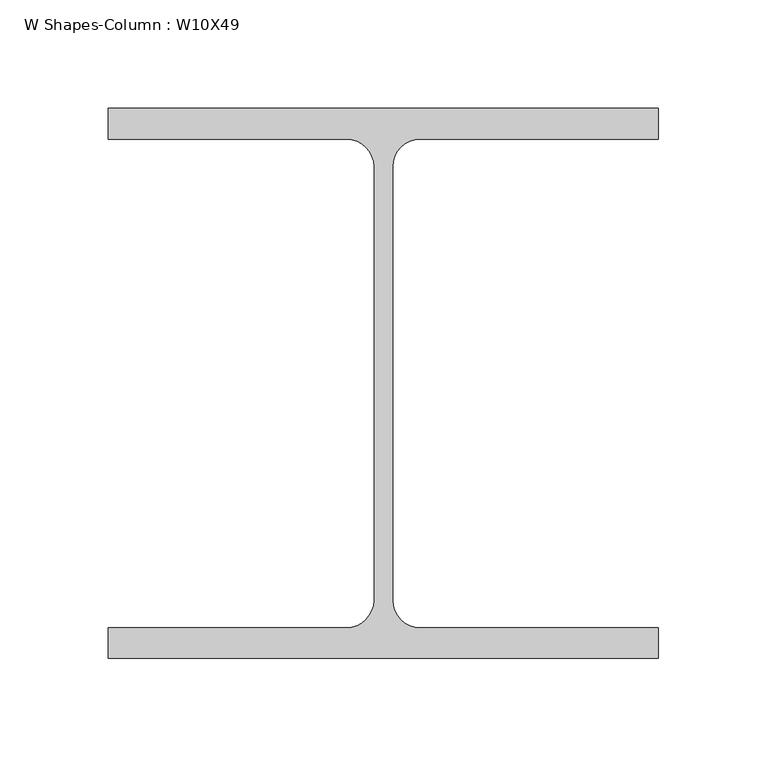
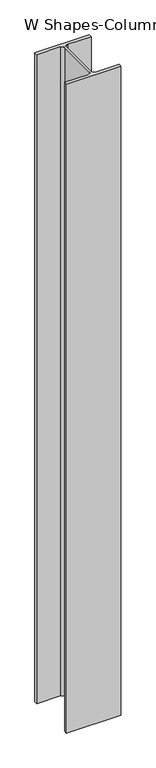
"""IFC4 building model written with IfcOpenShell, lengths in millimetres: column geometry, W Shapes-Column : W10X49."""

from ifc_helpers import new_model, si_unit, point, frame_2d, origin, origin_with_axes, place, context, project, spatial, polyline, circle_curve, trimmed, segment, composite_curve, outline, extrude, source, transform, mapped, element, save


def w_shapes_column_w10x49_27dd9c5e(model_context):
    return source(origin(), model_context, "Body", "SweptSolid", [
        extrude(outline(composite_curve([segment(polyline([(127.0, 127.0), (127.0, 112.776), (17.018, 112.776)]), True, "CONTINUOUS"), segment(trimmed(circle_curve(frame_2d((17.018, 100.076)), 12.7), [point((17.018, 112.776))], [point((4.318, 100.076))], True, "CARTESIAN"), True, "CONTINUOUS"), segment(polyline([(4.318, 100.076), (4.318, -100.076)]), True, "CONTINUOUS"), segment(trimmed(circle_curve(frame_2d((17.018, -100.076)), 12.7), [point((4.318, -100.076))], [point((17.018, -112.776))], True, "CARTESIAN"), True, "CONTINUOUS"), segment(polyline([(17.018, -112.776), (127.0, -112.776), (127.0, -127.0), (-127.0, -127.0), (-127.0, -112.776), (-17.018, -112.776)]), True, "CONTINUOUS"), segment(trimmed(circle_curve(frame_2d((-17.018, -100.076)), 12.7), [point((-17.018, -112.776))], [point((-4.318, -100.076))], True, "CARTESIAN"), True, "CONTINUOUS"), segment(polyline([(-4.318, -100.076), (-4.318, 100.076)]), True, "CONTINUOUS"), segment(trimmed(circle_curve(frame_2d((-17.018, 100.076)), 12.7), [point((-4.318, 100.076))], [point((-17.018, 112.776))], True, "CARTESIAN"), True, "CONTINUOUS"), segment(polyline([(-17.018, 112.776), (-127.0, 112.776), (-127.0, 127.0), (127.0, 127.0)]), True, "CONTINUOUS")], self_intersect=False)), origin_with_axes(), (0.0, 0.0, 1.0), 3200.4),
    ])


if __name__ == "__main__":
    model = new_model("IFC4")
    model_context = context("Model", 3, world=origin())
    ifc_project = project(units=[si_unit("LENGTHUNIT", "METRE", prefix="MILLI")], contexts=[model_context])
    site = spatial("IfcSite", under=ifc_project)
    building = spatial("IfcBuilding", under=site)
    placement = place(None, origin())
    w_shapes_column_w10x49_shape = w_shapes_column_w10x49_27dd9c5e(model_context)
    element("IfcColumn", 1, ObjectType="W Shapes-Column : W10X49", at=placement, inside=building, context=model_context, shape_type="MappedRepresentation", body=[
        mapped(w_shapes_column_w10x49_shape, transform((0.0, 0.0, 0.0), x_axis=(1.0, 0.0, 0.0), y_axis=(0.0, 1.0, 0.0), z_axis=(0.0, 0.0, 1.0))),
    ])
    save(model, "model.ifc")

# Revit data of these elements
# Type "W Shapes-Column : W10X49"
#   Section Name Key = "W10x49"
#   Assembly Code = "B10"
#   Width = 10.000"
#   Web Thickness = 0.340"
#   Web Fillet = 0.500"
#   Warping Constant = 2070.00 in⁶
#   Torsional Moment of Inertia = 1.39 in⁴
#   Section Area = 14.40 in²
#   Plastic Modulus weak axis = 28.30 in³
#   Plastic Modulus strong axis = 60.40 in³
#   Perimeter = 58.50 ft²/ft
#   Nominal Weight = 49.00 lbf/ft
#   Moment of Inertia weak axis = 93.40 in⁴
#   Moment of Inertia strong axis = 272.00 in⁴
#   Height = 10.000"
#   Flange Thickness = 0.560"
#   Elastic Modulus weak axis = 18.70 in³
#   Elastic Modulus strong axis = 54.60 in³
#   Centroid Vertical = 5.000"
#   Centroid Horizontal = 5.000"
#   Structural Material [instance default] = Steel ASTM A992
#   Principal Axes Angle = 0
# Element 1 (IfcColumn, "W Shapes-Column : W10X49")
#   Materials on its faces: "Steel ASTM A992"
# Materials
#   "Steel ASTM A992": class "Metal", colour RGB 199 199 199, transparency 0, Description = "Structural steel 50ksi", Cost = 0
